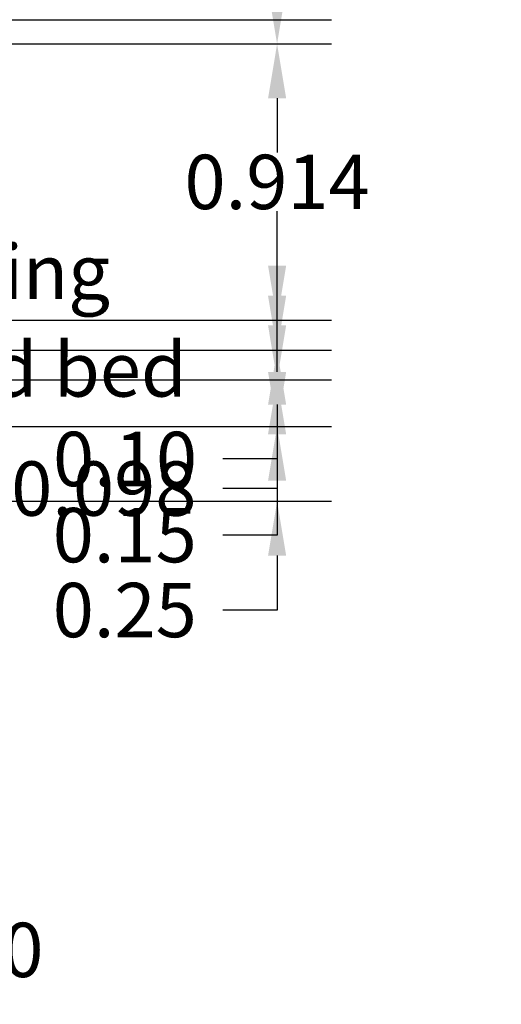
# Model space of a CAD drawing. Units: metres. Extents: x 22.1 to 34.4, y 4.4 to 12.4.
# Tile 7 of 8: x 32.8 to 34.4, y 6.2 to 9.5. Entities that reach past the tile are written whole.
import ezdxf
from ezdxf import colors
from ezdxf.entities.mleader import LeaderData, LeaderLine
from ezdxf.math import Vec2, Vec3

# ---------------------------------------------------------------- set-up
doc = ezdxf.new("R2010")
doc.units = ezdxf.units.M
doc.header["$MEASUREMENT"] = 0
for name, color, linetype, lineweight in [('A-ANNO-DIMS', 2, 'Continuous', 18), ('A-ANNO-TEXT', 7, 'Continuous', 18), ('C-TOPO', 3, 'Continuous', 25)]:
    doc.layers.add(name, color=color, linetype=linetype, lineweight=lineweight)
doc.styles.get("Standard").update_dxf_attribs({"font": 'arial.ttf'})
doc.dimstyles.get("Standard").update_dxf_attribs({"dimtxt": 0.18, "dimasz": 0.18, "dimexe": 0.18, "dimexo": 0.0625, "dimgap": 0.09, "dimtad": 0, "dimtih": 1, "dimtoh": 1, "dimzin": 0, "dimdsep": 46, "dimtxsty": 'Standard', "dimcen": 0.09, "dimadec": 0, "dimazin": 0, "dimtfac": 1, "dimtofl": 0, "dimtmove": 0, "dimatfit": 3, "dimfxl": 1, "dimtolj": 1, "dimtzin": 0, "dimarcsym": 0})

# ---------------------------------------------------------------- blocks, each defined once
blk = doc.blocks.new('*D18')
at = {"layer": 'A-ANNO-DIMS', "color": 0, "lineweight": -2, "transparency": 16777216}
for p, q in [((31.3118, 10.5649), (31.5885, 10.5649)), ((31.4085, 10.3849), (31.4085, 10.2175)), ((31.4085, 9.6839), (31.4085, 9.8513)), ((31.3118, 9.5039), (31.5885, 9.5039))]:
    blk.add_line(p, q, dxfattribs=at)
at = {"layer": 'A-ANNO-DIMS', "color": 0, "transparency": 16777216}
for points in [[(31.3785, 10.3849), (31.4385, 10.3849), (31.4085, 10.5649)], [(31.3785, 9.6839), (31.4385, 9.6839), (31.4085, 9.5039)]]:
    blk.add_solid(points, dxfattribs=at)
at = {"layer": 'Defpoints', "color": 0, "transparency": 16777216}
for p in [(31.2493, 10.5649), (31.4085, 10.5649), (31.2493, 9.5039)]:
    blk.add_point(p, dxfattribs=at)
at = {"layer": 'A-ANNO-DIMS', "color": 0, "transparency": 16777216, "insert": (31.4085, 10.0344), "char_height": 0.18, "attachment_point": 5}
blk.add_mtext('\\A1;WINDOW PANE 490 1.06 TYP.', dxfattribs=at)
blk = doc.blocks.new('*D28')
at = {"layer": 'A-ANNO-DIMS', "color": 0, "lineweight": -2, "transparency": 16777216}
for p, q in [((31.7781, 11.4474), (31.7781, 6.2449)), ((31.9781, 11.4474), (31.9781, 6.2449)), ((31.5981, 6.4249), (31.4181, 6.4249)), ((32.1581, 6.4249), (32.3381, 6.4249))]:
    blk.add_line(p, q, dxfattribs=at)
at = {"layer": 'A-ANNO-DIMS', "color": 0, "transparency": 16777216}
for points in [[(31.5981, 6.4549), (31.5981, 6.3949), (31.7781, 6.4249)], [(32.1581, 6.4549), (32.1581, 6.3949), (31.9781, 6.4249)]]:
    blk.add_solid(points, dxfattribs=at)
at = {"layer": 'Defpoints', "color": 0, "transparency": 16777216}
for p in [(31.7781, 11.5099), (31.9781, 11.5099), (31.9781, 6.4249)]:
    blk.add_point(p, dxfattribs=at)
at = {"layer": 'A-ANNO-DIMS', "color": 0, "transparency": 16777216, "insert": (32.6615, 6.4249), "char_height": 0.18, "attachment_point": 5}
blk.add_mtext('\\A1;0.20', dxfattribs=at)
blk = doc.blocks.new('*D40')
at = {"layer": 'A-ANNO-DIMS', "color": 0, "lineweight": -2, "transparency": 16777216}
for p, q in [((31.3918, 10.6399), (33.8537, 10.6399)), ((33.6737, 10.4599), (33.6737, 10.2138)), ((33.6737, 9.6039), (33.6737, 9.85)), ((31.3918, 9.4239), (33.8537, 9.4239))]:
    blk.add_line(p, q, dxfattribs=at)
at = {"layer": 'A-ANNO-DIMS', "color": 0, "transparency": 16777216}
for points in [[(33.6437, 10.4599), (33.7037, 10.4599), (33.6737, 10.6399)], [(33.6437, 9.6039), (33.7037, 9.6039), (33.6737, 9.4239)]]:
    blk.add_solid(points, dxfattribs=at)
at = {"layer": 'Defpoints', "color": 0, "transparency": 16777216}
for p in [(31.3293, 10.6399), (31.3293, 9.4239), (33.6737, 9.4239)]:
    blk.add_point(p, dxfattribs=at)
at = {"layer": 'A-ANNO-DIMS', "color": 0, "transparency": 16777216, "insert": (33.6737, 10.0319), "char_height": 0.18, "attachment_point": 5}
blk.add_mtext('\\A1;1.216', dxfattribs=at)
blk = doc.blocks.new('*D42')
at = {"layer": 'A-ANNO-DIMS', "color": 0, "lineweight": -2, "transparency": 16777216}
for p, q in [((33.6737, 9.6839), (33.6737, 9.8639)), ((33.6737, 9.8639), (33.8537, 9.8639)), ((31.3118, 9.5039), (33.8537, 9.5039)), ((31.3918, 9.4239), (33.8537, 9.4239)), ((33.6737, 9.2439), (33.6737, 9.0639))]:
    blk.add_line(p, q, dxfattribs=at)
at = {"layer": 'A-ANNO-DIMS', "color": 0, "transparency": 16777216}
for points in [[(33.6437, 9.6839), (33.7037, 9.6839), (33.6737, 9.5039)], [(33.6437, 9.2439), (33.7037, 9.2439), (33.6737, 9.4239)]]:
    blk.add_solid(points, dxfattribs=at)
at = {"layer": 'Defpoints', "color": 0, "transparency": 16777216}
for p in [(31.2493, 9.5039), (33.6737, 9.5039), (31.3293, 9.4239)]:
    blk.add_point(p, dxfattribs=at)
at = {"layer": 'A-ANNO-DIMS', "color": 0, "transparency": 16777216, "insert": (34.1776, 9.8639), "char_height": 0.18, "attachment_point": 5}
blk.add_mtext('\\A1;0.08', dxfattribs=at)
blk = doc.blocks.new('*D43')
at = {"layer": 'A-ANNO-DIMS', "color": 0, "lineweight": -2, "transparency": 16777216}
for p, q in [((31.3918, 9.4239), (33.8537, 9.4239)), ((33.6737, 9.2439), (33.6737, 9.1488)), ((33.6737, 8.6899), (33.6737, 8.785)), ((31.5706, 8.5099), (33.8537, 8.5099))]:
    blk.add_line(p, q, dxfattribs=at)
at = {"layer": 'A-ANNO-DIMS', "color": 0, "transparency": 16777216}
for points in [[(33.6437, 9.2439), (33.7037, 9.2439), (33.6737, 9.4239)], [(33.6437, 8.6899), (33.7037, 8.6899), (33.6737, 8.5099)]]:
    blk.add_solid(points, dxfattribs=at)
at = {"layer": 'Defpoints', "color": 0, "transparency": 16777216}
for p in [(31.3293, 9.4239), (31.5081, 8.5099), (33.6737, 8.5099)]:
    blk.add_point(p, dxfattribs=at)
at = {"layer": 'A-ANNO-DIMS', "color": 0, "transparency": 16777216, "insert": (33.6737, 8.9669), "char_height": 0.18, "attachment_point": 5}
blk.add_mtext('\\A1;0.914', dxfattribs=at)
blk = doc.blocks.new('*D44')
at = {"layer": 'A-ANNO-DIMS', "color": 0, "lineweight": -2, "transparency": 16777216}
for p, q in [((33.6737, 8.6899), (33.6737, 8.8699)), ((24.8474, 8.5099), (33.8537, 8.5099)), ((24.5474, 8.4099), (33.8537, 8.4099)), ((33.6737, 8.2299), (33.6737, 8.0499)), ((33.6737, 8.0499), (33.4937, 8.0499))]:
    blk.add_line(p, q, dxfattribs=at)
at = {"layer": 'A-ANNO-DIMS', "color": 0, "transparency": 16777216}
for points in [[(33.6437, 8.6899), (33.7037, 8.6899), (33.6737, 8.5099)], [(33.6437, 8.2299), (33.7037, 8.2299), (33.6737, 8.4099)]]:
    blk.add_solid(points, dxfattribs=at)
at = {"layer": 'Defpoints', "color": 0, "transparency": 16777216}
for p in [(24.7849, 8.5099), (24.4849, 8.4099), (33.6737, 8.4099)]:
    blk.add_point(p, dxfattribs=at)
at = {"layer": 'A-ANNO-DIMS', "color": 0, "transparency": 16777216, "insert": (33.1702, 8.0499), "char_height": 0.18, "attachment_point": 5}
blk.add_mtext('\\A1;0.10', dxfattribs=at)
blk = doc.blocks.new('*D45')
at = {"layer": 'A-ANNO-DIMS', "color": 0, "lineweight": -2, "transparency": 16777216}
for p, q in [((33.6737, 8.5899), (33.6737, 8.7699)), ((24.5474, 8.4099), (33.8537, 8.4099)), ((24.8474, 8.3119), (33.8537, 8.3119)), ((33.6737, 8.1319), (33.6737, 7.9519)), ((33.6737, 7.9519), (33.4937, 7.9519))]:
    blk.add_line(p, q, dxfattribs=at)
at = {"layer": 'A-ANNO-DIMS', "color": 0, "transparency": 16777216}
for points in [[(33.6437, 8.5899), (33.7037, 8.5899), (33.6737, 8.4099)], [(33.6437, 8.1319), (33.7037, 8.1319), (33.6737, 8.3119)]]:
    blk.add_solid(points, dxfattribs=at)
at = {"layer": 'Defpoints', "color": 0, "transparency": 16777216}
for p in [(24.4849, 8.4099), (24.7849, 8.3119), (33.6737, 8.3119)]:
    blk.add_point(p, dxfattribs=at)
at = {"layer": 'A-ANNO-DIMS', "color": 0, "transparency": 16777216, "insert": (33.0998, 7.9519), "char_height": 0.18, "attachment_point": 5}
blk.add_mtext('\\A1;0.098', dxfattribs=at)
blk = doc.blocks.new('*D46')
at = {"layer": 'A-ANNO-DIMS', "color": 0, "lineweight": -2, "transparency": 16777216}
for p, q in [((33.6737, 8.4919), (33.6737, 8.6719)), ((24.8474, 8.3119), (33.8537, 8.3119)), ((24.8474, 8.1578), (33.8537, 8.1578)), ((33.6737, 7.9778), (33.6737, 7.7978)), ((33.6737, 7.7978), (33.4937, 7.7978))]:
    blk.add_line(p, q, dxfattribs=at)
at = {"layer": 'A-ANNO-DIMS', "color": 0, "transparency": 16777216}
for points in [[(33.6437, 8.4919), (33.7037, 8.4919), (33.6737, 8.3119)], [(33.6437, 7.9778), (33.7037, 7.9778), (33.6737, 8.1578)]]:
    blk.add_solid(points, dxfattribs=at)
at = {"layer": 'Defpoints', "color": 0, "transparency": 16777216}
for p in [(24.7849, 8.3119), (24.7849, 8.1578), (33.6737, 8.1578)]:
    blk.add_point(p, dxfattribs=at)
at = {"layer": 'A-ANNO-DIMS', "color": 0, "transparency": 16777216, "insert": (33.1692, 7.7978), "char_height": 0.18, "attachment_point": 5}
blk.add_mtext('\\A1;0.15', dxfattribs=at)
blk = doc.blocks.new('*D47')
at = {"layer": 'A-ANNO-DIMS', "color": 0, "lineweight": -2, "transparency": 16777216}
for p, q in [((33.6737, 8.3378), (33.6737, 8.5178)), ((24.8474, 8.1578), (33.8537, 8.1578)), ((24.8474, 7.9099), (33.8537, 7.9099)), ((33.6737, 7.7299), (33.6737, 7.5499)), ((33.6737, 7.5499), (33.4937, 7.5499))]:
    blk.add_line(p, q, dxfattribs=at)
at = {"layer": 'A-ANNO-DIMS', "color": 0, "transparency": 16777216}
for points in [[(33.6437, 8.3378), (33.7037, 8.3378), (33.6737, 8.1578)], [(33.6437, 7.7299), (33.7037, 7.7299), (33.6737, 7.9099)]]:
    blk.add_solid(points, dxfattribs=at)
at = {"layer": 'Defpoints', "color": 0, "transparency": 16777216}
for p in [(24.7849, 8.1578), (24.7849, 7.9099), (33.6737, 7.9099)]:
    blk.add_point(p, dxfattribs=at)
at = {"layer": 'A-ANNO-DIMS', "color": 0, "transparency": 16777216, "insert": (33.1692, 7.5499), "char_height": 0.18, "attachment_point": 5}
blk.add_mtext('\\A1;0.25', dxfattribs=at)

msp = doc.modelspace()

# ---------------------------------------------------------------- linework, layer by layer
at = {"layer": 'C-TOPO'}
msp.add_line((31.9081, 7.9099), (33.0887, 7.9099), dxfattribs=at)

# ---------------------------------------------------------------- dimensions: what is measured, and where the dimension line sits
at = {"layer": 'A-ANNO-DIMS'}
dim = msp.add_linear_dim(base=(31.9781, 6.4249), p1=(31.7781, 11.5099), p2=(31.9781, 11.5099), dimstyle='Standard', override={"dimdec": 2, "dimlfac": 1, "dimrnd": 0, "dimzin": 0, "dimdsep": 46, "dimlunit": 2}, dxfattribs=at)
dim.commit()
dim.dimension.update_dxf_attribs({"geometry": '*D28', "text_midpoint": (32.6615, 6.4249)})
dim = msp.add_linear_dim(base=(31.4085, 10.5649), p1=(31.2493, 9.5039), p2=(31.2493, 10.5649), angle=90, text='WINDOW PANE 490 <> TYP.', dimstyle='Standard', override={"dimdec": 2, "dimrnd": 0, "dimzin": 0, "dimlunit": 2}, dxfattribs=at)
dim.commit()
dim.dimension.update_dxf_attribs({"geometry": '*D18', "text_midpoint": (31.4085, 10.0344)})
for base, p1, p2, override, picture, middle in [((33.6737, 9.4239), (31.3293, 10.6399), (31.3293, 9.4239), {"dimdec": 3, "dimlfac": 1, "dimrnd": 0, "dimzin": 0, "dimdsep": 46, "dimlunit": 2}, '*D40', (33.6737, 10.0319)), ((33.6737, 9.5039), (31.3293, 9.4239), (31.2493, 9.5039), {"dimdec": 2, "dimlfac": 1, "dimrnd": 0, "dimzin": 0, "dimdsep": 46, "dimlunit": 2}, '*D42', (34.1776, 9.8639)), ((33.6737, 8.5099), (31.3293, 9.4239), (31.5081, 8.5099), {"dimdec": 3, "dimlfac": 1, "dimrnd": 0, "dimzin": 0, "dimdsep": 46, "dimlunit": 2}, '*D43', (33.6737, 8.9669)), ((33.6737, 8.4099), (24.7849, 8.5099), (24.4849, 8.4099), {"dimdec": 2, "dimlfac": 1, "dimrnd": 0, "dimzin": 0, "dimdsep": 46, "dimlunit": 2}, '*D44', (33.1702, 8.0499)), ((33.6737, 8.3119), (24.4849, 8.4099), (24.7849, 8.3119), {"dimdec": 3, "dimlfac": 1, "dimrnd": 0, "dimzin": 0, "dimdsep": 46, "dimlunit": 2}, '*D45', (33.0998, 7.9519)), ((33.6737, 8.1578), (24.7849, 8.3119), (24.7849, 8.1578), {"dimdec": 2, "dimlfac": 1, "dimrnd": 0, "dimzin": 0, "dimdsep": 46, "dimlunit": 2}, '*D46', (33.1692, 7.7978)), ((33.6737, 7.9099), (24.7849, 8.1578), (24.7849, 7.9099), {"dimdec": 2, "dimlfac": 1, "dimrnd": 0, "dimzin": 0, "dimdsep": 46, "dimlunit": 2}, '*D47', (33.1692, 7.5499))]:
    dim = msp.add_linear_dim(base=base, p1=p1, p2=p2, angle=90, dimstyle='Standard', override=override, dxfattribs=at)
    dim.commit()
    dim.dimension.update_dxf_attribs({"geometry": picture, "text_midpoint": middle})

# ---------------------------------------------------------------- leaders
at = {"layer": 'A-ANNO-TEXT'}
ml = msp.add_multileader_mtext('Standard', dxfattribs=at)
ml.set_content('Coping', color=256)
ml.set_leader_properties()
ml.build(insert=Vec2(0, 0))
ml.multileader.update_dxf_attribs({"dogleg_length": 0.36, "arrow_head_size": 0.18})
ctx = ml.context
ctx.base_point, ctx.char_height, ctx.arrow_head_size, ctx.landing_gap_size, ctx.plane_origin = Vec3(32.2169, 8.6432), 0.18, 0.18, 0.09, Vec3(31.6868, 8.4551)
notes = []
notes.append((ctx, [(0, (1, 1, 0), (32.0498, 8.6432), (1, 0), 0.1671, [(0, [(31.6868, 8.4551)], 0, [])])]))
ctx.mtext.insert, ctx.mtext.flow_direction = Vec3(32.3069, 8.7596), 5
ml = msp.add_multileader_mtext('Standard', dxfattribs=at)
ml.set_content('Sand bed', color=256)
ml.set_leader_properties()
ml.build(insert=Vec2(0, 0))
ml.multileader.update_dxf_attribs({"dogleg_length": 0.36, "arrow_head_size": 0.18})
ctx = ml.context
ctx.base_point, ctx.char_height, ctx.arrow_head_size, ctx.landing_gap_size, ctx.plane_origin = Vec3(32.2032, 8.3447), 0.18, 0.18, 0.09, Vec3(31.4464, 8.3479)
notes.append((ctx, [(0, (1, 1, 0), (32.0951, 8.3447), (1, 0), 0.1082, [(0, [(31.4464, 8.3479)], 0, [])])]))
ctx.mtext.insert, ctx.mtext.flow_direction = Vec3(32.2932, 8.4363), 5
for ctx, leaders in notes:
    for number, flags, end, landing, length, lines in leaders:
        leader = LeaderData()
        leader.index, (leader.has_last_leader_line, leader.has_dogleg_vector, leader.attachment_direction) = number, flags
        leader.last_leader_point, leader.dogleg_vector, leader.dogleg_length = Vec3(end), Vec3(landing), length
        for number, points, colour, breaks in lines:
            line = LeaderLine()
            line.index, line.vertices, line.color, line.breaks = number, Vec3.list(points), colors.encode_raw_color(colour), breaks
            leader.lines.append(line)
        ctx.leaders.append(leader)

doc.saveas('drawing.dxf')
